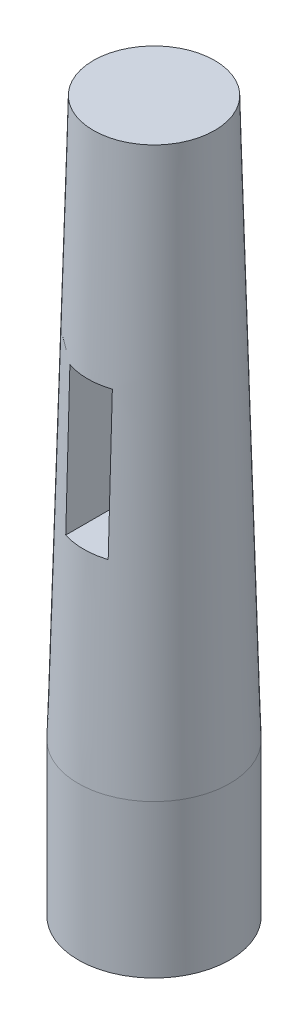
from build123d import *

# Parameters (mm, degrees)
BASE_SHANK_PROFILE_25_2_R  = 12.5
BASE_SHANK_25_2_DEPTH      = 25.2
TAPER_START_PROFILE_25_2_R = 12.5
TAPER_END_PROFILE_20_2_R   = 10
THROUGH_SLOT_PROFILE_W     = 7
THROUGH_SLOT_PROFILE_H     = 24
THROUGH_SLOT_DEPTH         = 17.6


with BuildPart() as part:
    # Base Shank Profile Ø25.2 → Base Shank Ø25.2 (new body)
    with BuildSketch(Plane(origin=(0, 0, 0), x_dir=(1, 0, 0), z_dir=(0, 1, 0))):
        with Locations(Location((0, 0, 0), (0, 0, 270))):
            Circle(BASE_SHANK_PROFILE_25_2_R)
    extrude(amount=BASE_SHANK_25_2_DEPTH)

    # Taper Start Profile Ø25.2 → Tapered Rod Loft section 0
    with BuildSketch(Plane(origin=(0, 25.2, 0), x_dir=(1, 0, 0), z_dir=(0, 1, 0))):
        Circle(TAPER_START_PROFILE_25_2_R)
    # Taper End Profile Ø20.2 → Tapered Rod Loft section 1
    with BuildSketch(Plane(origin=(0, 117.2, 0), x_dir=(1, 0, 0), z_dir=(0, 1, 0))):
        Circle(TAPER_END_PROFILE_20_2_R)
    loft()

    # Through Slot Profile → Through Slot (cut, symmetric)
    with BuildSketch(Plane.XY):
        with Locations((0, 70.2)):
            Rectangle(THROUGH_SLOT_PROFILE_W, THROUGH_SLOT_PROFILE_H)
    extrude(amount=THROUGH_SLOT_DEPTH, both=True, mode=Mode.SUBTRACT)


solid = part.part
